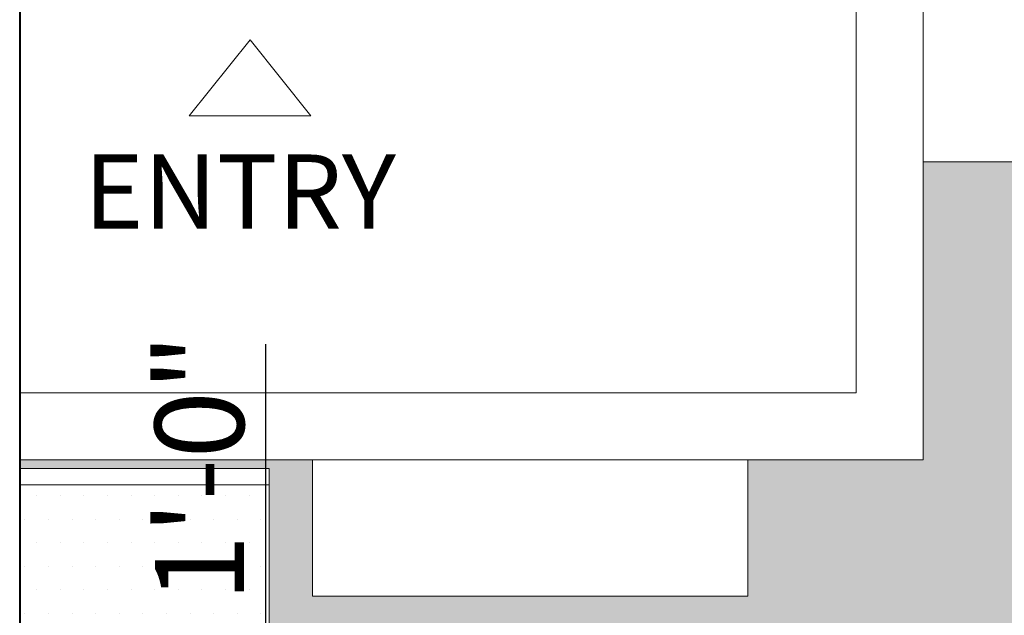
# Model space of a CAD drawing. Units: inches. Extents: x 459864 to 460310, y 324185 to 324787.
# Tile 44 of 112: x 460061 to 460127, y 324242 to 324282. Entities that reach past the tile are written whole.
import ezdxf

# ---------------------------------------------------------------- set-up
doc = ezdxf.new("R2010")
doc.units = ezdxf.units.IN
for name, color, linetype, lineweight in [('A-ANNO-DIMS', 2, 'Continuous', 18), ('A-ANNO-SYMB', 7, 'Continuous', 18), ('A-ANNO-TEXT', 7, 'Continuous', 18), ('A-WALL', 7, 'Continuous', 40), ('L-HRDS', 9, 'Continuous', 18), ('L-PLNT', 3, 'Continuous', 13), ('L-SITE-PATT', 252, 'Continuous', 13)]:
    doc.layers.add(name, color=color, linetype=linetype, lineweight=lineweight)
doc.styles.get("Standard").update_dxf_attribs({"font": 'arial.ttf'})
doc.dimstyles.new('ISO-25', dxfattribs={"dimtxt": 6, "dimasz": 2.5, "dimexe": 1.25, "dimexo": 0.625, "dimtad": 1, "dimdec": 1, "dimlunit": 3, "dimtxsty": 'Standard', "dimcen": 2.5, "dimadec": 0, "dimazin": 0, "dimtfac": 1, "dimtdec": 1, "dimtmove": 0, "dimatfit": 3, "dimfxl": 1, "dimarcsym": 0})

# ---------------------------------------------------------------- blocks, each defined once
blk = doc.blocks.new('*D28')
at = {"layer": 'A-ANNO-DIMS', "color": 0, "lineweight": -2, "transparency": 16777216}
for p, q in [((460148.65, 324370.7), (460136.025, 324370.7)), ((460137.275, 324368.2), (460137.275, 324293.2)), ((460148.65, 324290.7), (460136.025, 324290.7)), ((460137.275, 324290.7), (460137.275, 324198.69))]:
    blk.add_line(p, q, dxfattribs=at)
at = {"layer": 'A-ANNO-DIMS', "color": 0, "transparency": 16777216}
for points in [[(460136.858, 324368.2), (460137.692, 324368.2), (460137.275, 324370.7)], [(460136.858, 324293.2), (460137.692, 324293.2), (460137.275, 324290.7)]]:
    blk.add_solid(points, dxfattribs=at)
at = {"layer": 'Defpoints', "color": 0, "transparency": 16777216}
for p in [(460149.275, 324370.7), (460137.275, 324290.7), (460149.275, 324290.7)]:
    blk.add_point(p, dxfattribs=at)
at = {"layer": 'A-ANNO-DIMS', "color": 0, "transparency": 16777216, "insert": (460133.363, 324243.445), "char_height": 6, "attachment_point": 5, "rotation": 90}
blk.add_mtext('QUEEN BED 6\'-8" TYP.', dxfattribs=at)
blk = doc.blocks.new('*D37')
at = {"layer": 'A-ANNO-DIMS', "color": 0, "lineweight": -2, "transparency": 16777216}
for p, q in [((460077.678, 324241.122), (460077.678, 324260.257)), ((460076.501, 324241.122), (460078.928, 324241.122)), ((460077.678, 324231.608), (460077.678, 324238.622)), ((460076.501, 324229.108), (460078.928, 324229.108))]:
    blk.add_line(p, q, dxfattribs=at)
at = {"layer": 'A-ANNO-DIMS', "color": 0, "transparency": 16777216}
for points in [[(460077.261, 324238.622), (460078.095, 324238.622), (460077.678, 324241.122)], [(460077.261, 324231.608), (460078.095, 324231.608), (460077.678, 324229.108)]]:
    blk.add_solid(points, dxfattribs=at)
at = {"layer": 'Defpoints', "color": 0, "transparency": 16777216}
for p in [(460075.876, 324241.122), (460077.678, 324241.122), (460075.876, 324229.108)]:
    blk.add_point(p, dxfattribs=at)
at = {"layer": 'A-ANNO-DIMS', "color": 0, "transparency": 16777216, "insert": (460073.989, 324251.94), "char_height": 6, "attachment_point": 5, "rotation": 90}
blk.add_mtext('1\'-0"', dxfattribs=at)

msp = doc.modelspace()

# ---------------------------------------------------------------- hatches: boundary and pattern name
at = {"layer": 'L-SITE-PATT'}
h = msp.add_hatch(dxfattribs=at)
h.set_pattern_fill('DOTS', color=256)
h.paths.add_polyline_path([(460269.804, 324283.483), (460247.115, 324283.483), (460121.929, 324283.483), (460121.929, 324252.473), (460117.429, 324252.473), (460110.124, 324252.473), (460110.124, 324243.287), (460080.83, 324243.287), (460080.83, 324252.473), (460061.115, 324252.473), (460061.115, 324251.882), (460077.909, 324251.882), (460077.909, 324199.483), (460080.83, 324199.483), (460080.83, 324207.553), (460110.124, 324207.553), (460110.124, 324199.483), (460110.813, 324199.483), (460262.115, 324199.483), (460269.804, 324199.483)], flags=17)
edge = h.paths.add_edge_path(flags=0)
edge.add_ellipse((460222.59, 324263.813), major_axis=(-8.485, 8.485), ratio=1, start_angle=405, end_angle=495, ccw=False)
edge.add_line((460214.821, 324254.66), (460214.832, 324254.666))
edge.add_ellipse((460222.59, 324263.813), major_axis=(-8.485, 8.485), ratio=1, start_angle=405, end_angle=495, ccw=False)
edge.add_line((460210.759, 324261.781), (460210.768, 324261.787))
edge.add_ellipse((460222.59, 324263.813), major_axis=(-8.485, 8.485), ratio=1, start_angle=405, end_angle=495, ccw=False)
edge.add_ellipse((460222.59, 324263.813), major_axis=(-8.485, 8.485), ratio=1, start_angle=392.75402, end_angle=405, ccw=False)
edge.add_ellipse((460222.59, 324263.813), major_axis=(-8.485, 8.485), ratio=1, start_angle=380.93472, end_angle=392.75402, ccw=False)
edge.add_line((460211.337, 324267.985), (460211.34, 324267.985))
edge.add_ellipse((460222.59, 324263.813), major_axis=(-8.485, 8.485), ratio=1, start_angle=380.93472, end_angle=392.75402, ccw=False)
edge.add_ellipse((460222.59, 324263.813), major_axis=(-8.485, 8.485), ratio=1, start_angle=347.90152, end_angle=380.93472, ccw=False)
edge.add_ellipse((460222.59, 324263.813), major_axis=(-8.485, 8.485), ratio=1, start_angle=327.06192, end_angle=347.90152, ccw=False)
edge.add_ellipse((460222.59, 324263.813), major_axis=(-8.485, 8.485), ratio=1, start_angle=278.32464, end_angle=327.06192, ccw=False)
edge.add_line((460225.158, 324275.536), (460225.158, 324275.535))
edge.add_ellipse((460222.59, 324263.813), major_axis=(-8.485, 8.485), ratio=1, start_angle=278.32464, end_angle=327.06192, ccw=False)
edge.add_ellipse((460222.59, 324263.813), major_axis=(-8.485, 8.485), ratio=1, start_angle=260.64357, end_angle=278.32464, ccw=False)
edge.add_ellipse((460222.59, 324263.813), major_axis=(-8.485, 8.485), ratio=1, start_angle=225, end_angle=260.64357, ccw=False)
edge.add_line((460234.509, 324265.243), (460234.501, 324265.239))
edge.add_ellipse((460222.59, 324263.813), major_axis=(-8.485, 8.485), ratio=1, start_angle=225, end_angle=260.64357, ccw=False)
edge.add_ellipse((460222.59, 324263.813), major_axis=(-8.485, 8.485), ratio=1, start_angle=495, end_angle=585, ccw=False)
edge.add_line((460234.437, 324261.861), (460234.424, 324261.858))
edge.add_ellipse((460222.59, 324263.813), major_axis=(-8.485, 8.485), ratio=1, start_angle=495, end_angle=585, ccw=False)
edge.add_line((460227.95, 324253.067), (460227.946, 324253.083))
edge.add_ellipse((460222.59, 324263.813), major_axis=(-8.485, 8.485), ratio=1, start_angle=495, end_angle=585, ccw=False)
edge.add_line((460226.223, 324252.369), (460226.211, 324252.38))
edge.add_ellipse((460222.59, 324263.813), major_axis=(-8.485, 8.485), ratio=1, start_angle=495, end_angle=585, ccw=False)
h.paths.add_polyline_path([(460219.651, 324254.347), (460218.461, 324253.545), (460218.275, 324254.789), (460219.642, 324256.542), (460219.625, 324260.848), (460216.11, 324257.333), (460214.35, 324256.978), (460215.416, 324259.356), (460212.524, 324258.496), (460213.137, 324259.93), (460218.507, 324263.813), (460222.59, 324263.813), (460222.59, 324267.807), (460218.176, 324272.212), (460219.026, 324274.639), (460222.59, 324272.811), (460222.59, 324275.423), (460223.057, 324274.825), (460222.675, 324273.492), (460225.912, 324267.135), (460219.625, 324260.848)], flags=0)
edge = h.paths.add_edge_path(flags=0)
edge.add_ellipse((460194.576, 324264.046), major_axis=(-8.485, 8.485), ratio=1, start_angle=495, end_angle=585, ccw=False)
edge.add_line((460199.936, 324253.3), (460199.932, 324253.316))
edge.add_ellipse((460194.576, 324264.046), major_axis=(-8.485, 8.485), ratio=1, start_angle=495, end_angle=585, ccw=False)
edge.add_line((460198.208, 324252.603), (460198.196, 324252.613))
edge.add_ellipse((460194.576, 324264.046), major_axis=(-8.485, 8.485), ratio=1, start_angle=495, end_angle=585, ccw=False)
edge.add_ellipse((460194.576, 324264.046), major_axis=(-8.485, 8.485), ratio=1, start_angle=405, end_angle=495, ccw=False)
edge.add_line((460186.806, 324254.893), (460186.817, 324254.899))
edge.add_ellipse((460194.576, 324264.046), major_axis=(-8.485, 8.485), ratio=1, start_angle=405, end_angle=495, ccw=False)
edge.add_line((460182.744, 324262.014), (460182.753, 324262.02))
edge.add_ellipse((460194.576, 324264.046), major_axis=(-8.485, 8.485), ratio=1, start_angle=405, end_angle=495, ccw=False)
edge.add_ellipse((460194.576, 324264.046), major_axis=(-8.485, 8.485), ratio=1, start_angle=392.75402, end_angle=405, ccw=False)
edge.add_ellipse((460194.576, 324264.046), major_axis=(-8.485, 8.485), ratio=1, start_angle=380.93472, end_angle=392.75402, ccw=False)
edge.add_line((460183.323, 324268.218), (460183.326, 324268.218))
edge.add_ellipse((460194.576, 324264.046), major_axis=(-8.485, 8.485), ratio=1, start_angle=380.93472, end_angle=392.75402, ccw=False)
edge.add_ellipse((460194.576, 324264.046), major_axis=(-8.485, 8.485), ratio=1, start_angle=347.90152, end_angle=380.93472, ccw=False)
edge.add_ellipse((460194.576, 324264.046), major_axis=(-8.485, 8.485), ratio=1, start_angle=327.06192, end_angle=347.90152, ccw=False)
edge.add_ellipse((460194.576, 324264.046), major_axis=(-8.485, 8.485), ratio=1, start_angle=278.32464, end_angle=327.06192, ccw=False)
edge.add_line((460197.144, 324275.769), (460197.143, 324275.768))
edge.add_ellipse((460194.576, 324264.046), major_axis=(-8.485, 8.485), ratio=1, start_angle=278.32464, end_angle=327.06192, ccw=False)
edge.add_ellipse((460194.576, 324264.046), major_axis=(-8.485, 8.485), ratio=1, start_angle=260.64357, end_angle=278.32464, ccw=False)
edge.add_ellipse((460194.576, 324264.046), major_axis=(-8.485, 8.485), ratio=1, start_angle=225, end_angle=260.64357, ccw=False)
edge.add_line((460206.494, 324265.476), (460206.487, 324265.473))
edge.add_ellipse((460194.576, 324264.046), major_axis=(-8.485, 8.485), ratio=1, start_angle=225, end_angle=260.64357, ccw=False)
edge.add_ellipse((460194.576, 324264.046), major_axis=(-8.485, 8.485), ratio=1, start_angle=495, end_angle=585, ccw=False)
edge.add_line((460206.422, 324262.094), (460206.409, 324262.091))
h.paths.add_polyline_path([(460191.61, 324261.081), (460191.637, 324254.58), (460190.447, 324253.778), (460190.261, 324255.023), (460191.628, 324256.775), (460191.61, 324261.081), (460188.096, 324257.566), (460186.335, 324257.211), (460187.402, 324259.589), (460184.509, 324258.729), (460185.123, 324260.163), (460190.493, 324264.046), (460194.576, 324264.046), (460194.576, 324268.04), (460190.161, 324272.446), (460191.011, 324274.872), (460194.576, 324273.044), (460194.576, 324275.657), (460195.043, 324275.058), (460194.661, 324273.725), (460197.897, 324267.368)], flags=0)
edge = h.paths.add_edge_path(flags=0)
edge.add_ellipse((460252.912, 324263.578), major_axis=(-8.485, 8.485), ratio=1, start_angle=405, end_angle=495, ccw=False)
edge.add_line((460241.081, 324261.545), (460241.089, 324261.551))
edge.add_ellipse((460252.912, 324263.578), major_axis=(-8.485, 8.485), ratio=1, start_angle=405, end_angle=495, ccw=False)
edge.add_ellipse((460252.912, 324263.578), major_axis=(-8.485, 8.485), ratio=1, start_angle=392.75402, end_angle=405, ccw=False)
edge.add_ellipse((460252.912, 324263.578), major_axis=(-8.485, 8.485), ratio=1, start_angle=380.93472, end_angle=392.75402, ccw=False)
edge.add_line((460241.659, 324267.749), (460241.662, 324267.749))
edge.add_ellipse((460252.912, 324263.578), major_axis=(-8.485, 8.485), ratio=1, start_angle=380.93472, end_angle=392.75402, ccw=False)
edge.add_ellipse((460252.912, 324263.578), major_axis=(-8.485, 8.485), ratio=1, start_angle=347.90152, end_angle=380.93472, ccw=False)
edge.add_ellipse((460252.912, 324263.578), major_axis=(-8.485, 8.485), ratio=1, start_angle=327.06192, end_angle=347.90152, ccw=False)
edge.add_ellipse((460252.912, 324263.578), major_axis=(-8.485, 8.485), ratio=1, start_angle=278.32464, end_angle=327.06192, ccw=False)
edge.add_line((460255.48, 324275.3), (460255.479, 324275.299))
edge.add_ellipse((460252.912, 324263.578), major_axis=(-8.485, 8.485), ratio=1, start_angle=278.32464, end_angle=327.06192, ccw=False)
edge.add_ellipse((460252.912, 324263.578), major_axis=(-8.485, 8.485), ratio=1, start_angle=260.64357, end_angle=278.32464, ccw=False)
edge.add_ellipse((460252.912, 324263.578), major_axis=(-8.485, 8.485), ratio=1, start_angle=225, end_angle=260.64357, ccw=False)
edge.add_line((460264.83, 324265.007), (460264.823, 324265.004))
edge.add_ellipse((460252.912, 324263.578), major_axis=(-8.485, 8.485), ratio=1, start_angle=225, end_angle=260.64357, ccw=False)
edge.add_ellipse((460252.912, 324263.578), major_axis=(-8.485, 8.485), ratio=1, start_angle=495, end_angle=585, ccw=False)
edge.add_line((460264.758, 324261.626), (460264.745, 324261.622))
edge.add_ellipse((460252.912, 324263.578), major_axis=(-8.485, 8.485), ratio=1, start_angle=495, end_angle=585, ccw=False)
edge.add_line((460258.272, 324252.832), (460258.268, 324252.848))
edge.add_ellipse((460252.912, 324263.578), major_axis=(-8.485, 8.485), ratio=1, start_angle=495, end_angle=585, ccw=False)
edge.add_line((460256.545, 324252.134), (460256.533, 324252.144))
edge.add_ellipse((460252.912, 324263.578), major_axis=(-8.485, 8.485), ratio=1, start_angle=495, end_angle=585, ccw=False)
edge.add_ellipse((460252.912, 324263.578), major_axis=(-8.485, 8.485), ratio=1, start_angle=405, end_angle=495, ccw=False)
edge.add_line((460245.143, 324254.424), (460245.153, 324254.43))
h.paths.add_polyline_path([(460244.672, 324256.742), (460245.738, 324259.12), (460242.846, 324258.26), (460243.459, 324259.694), (460248.829, 324263.578), (460252.912, 324263.578), (460252.912, 324267.571), (460248.497, 324271.977), (460249.348, 324274.403), (460252.912, 324272.576), (460252.912, 324275.188), (460253.379, 324274.589), (460252.997, 324273.257), (460256.233, 324266.899), (460249.946, 324260.612), (460249.973, 324254.111), (460248.783, 324253.309), (460248.597, 324254.554), (460249.964, 324256.306), (460249.946, 324260.612), (460246.432, 324257.097)], flags=0)
edge = h.paths.add_edge_path(flags=0)
edge.add_ellipse((460167.439, 324262.833), major_axis=(-8.485, 8.485), ratio=1, start_angle=495, end_angle=585, ccw=False)
edge.add_line((460172.799, 324252.087), (460172.795, 324252.103))
edge.add_ellipse((460167.439, 324262.833), major_axis=(-8.485, 8.485), ratio=1, start_angle=495, end_angle=585, ccw=False)
edge.add_line((460171.071, 324251.389), (460171.059, 324251.399))
edge.add_ellipse((460167.439, 324262.833), major_axis=(-8.485, 8.485), ratio=1, start_angle=495, end_angle=585, ccw=False)
edge.add_ellipse((460167.439, 324262.833), major_axis=(-8.485, 8.485), ratio=1, start_angle=405, end_angle=495, ccw=False)
edge.add_line((460159.669, 324253.679), (460159.68, 324253.685))
edge.add_ellipse((460167.439, 324262.833), major_axis=(-8.485, 8.485), ratio=1, start_angle=405, end_angle=495, ccw=False)
edge.add_line((460155.607, 324260.8), (460155.616, 324260.806))
edge.add_ellipse((460167.439, 324262.833), major_axis=(-8.485, 8.485), ratio=1, start_angle=405, end_angle=495, ccw=False)
edge.add_ellipse((460167.439, 324262.833), major_axis=(-8.485, 8.485), ratio=1, start_angle=392.75402, end_angle=405, ccw=False)
edge.add_ellipse((460167.439, 324262.833), major_axis=(-8.485, 8.485), ratio=1, start_angle=380.93472, end_angle=392.75402, ccw=False)
edge.add_line((460156.185, 324267.005), (460156.189, 324267.005))
edge.add_ellipse((460167.439, 324262.833), major_axis=(-8.485, 8.485), ratio=1, start_angle=380.93472, end_angle=392.75402, ccw=False)
edge.add_ellipse((460167.439, 324262.833), major_axis=(-8.485, 8.485), ratio=1, start_angle=347.90152, end_angle=380.93472, ccw=False)
edge.add_ellipse((460167.439, 324262.833), major_axis=(-8.485, 8.485), ratio=1, start_angle=327.06192, end_angle=347.90152, ccw=False)
edge.add_ellipse((460167.439, 324262.833), major_axis=(-8.485, 8.485), ratio=1, start_angle=278.32464, end_angle=327.06192, ccw=False)
edge.add_line((460170.007, 324274.556), (460170.006, 324274.554))
edge.add_ellipse((460167.439, 324262.833), major_axis=(-8.485, 8.485), ratio=1, start_angle=278.32464, end_angle=327.06192, ccw=False)
edge.add_ellipse((460167.439, 324262.833), major_axis=(-8.485, 8.485), ratio=1, start_angle=260.64357, end_angle=278.32464, ccw=False)
edge.add_ellipse((460167.439, 324262.833), major_axis=(-8.485, 8.485), ratio=1, start_angle=225, end_angle=260.64357, ccw=False)
edge.add_line((460179.357, 324264.262), (460179.35, 324264.259))
edge.add_ellipse((460167.439, 324262.833), major_axis=(-8.485, 8.485), ratio=1, start_angle=225, end_angle=260.64357, ccw=False)
edge.add_ellipse((460167.439, 324262.833), major_axis=(-8.485, 8.485), ratio=1, start_angle=495, end_angle=585, ccw=False)
edge.add_line((460179.285, 324260.881), (460179.272, 324260.877))
h.paths.add_polyline_path([(460164.473, 324259.867), (460164.5, 324253.366), (460163.31, 324252.565), (460163.124, 324253.809), (460164.491, 324255.561), (460164.473, 324259.867), (460160.958, 324256.353), (460159.198, 324255.998), (460160.265, 324258.375), (460157.372, 324257.515), (460157.986, 324258.949), (460163.356, 324262.833), (460167.439, 324262.833), (460167.439, 324266.826), (460163.024, 324271.232), (460163.874, 324273.659), (460167.439, 324271.831), (460167.439, 324274.443), (460167.905, 324273.844), (460167.524, 324272.512), (460170.76, 324266.154)], flags=0)
edge = h.paths.add_edge_path(flags=0)
edge.add_ellipse((460140.758, 324262.37), major_axis=(-8.485, 8.485), ratio=1, start_angle=495, end_angle=585, ccw=False)
edge.add_line((460146.118, 324251.624), (460146.114, 324251.639))
edge.add_ellipse((460140.758, 324262.37), major_axis=(-8.485, 8.485), ratio=1, start_angle=495, end_angle=585, ccw=False)
edge.add_line((460144.391, 324250.926), (460144.379, 324250.936))
edge.add_ellipse((460140.758, 324262.37), major_axis=(-8.485, 8.485), ratio=1, start_angle=495, end_angle=585, ccw=False)
edge.add_ellipse((460140.758, 324262.37), major_axis=(-8.485, 8.485), ratio=1, start_angle=405, end_angle=495, ccw=False)
edge.add_line((460132.989, 324253.216), (460132.999, 324253.222))
edge.add_ellipse((460140.758, 324262.37), major_axis=(-8.485, 8.485), ratio=1, start_angle=405, end_angle=495, ccw=False)
edge.add_line((460128.927, 324260.337), (460128.935, 324260.343))
edge.add_ellipse((460140.758, 324262.37), major_axis=(-8.485, 8.485), ratio=1, start_angle=405, end_angle=495, ccw=False)
edge.add_ellipse((460140.758, 324262.37), major_axis=(-8.485, 8.485), ratio=1, start_angle=392.75402, end_angle=405, ccw=False)
edge.add_ellipse((460140.758, 324262.37), major_axis=(-8.485, 8.485), ratio=1, start_angle=380.93472, end_angle=392.75402, ccw=False)
edge.add_line((460129.505, 324266.541), (460129.508, 324266.541))
edge.add_ellipse((460140.758, 324262.37), major_axis=(-8.485, 8.485), ratio=1, start_angle=380.93472, end_angle=392.75402, ccw=False)
edge.add_ellipse((460140.758, 324262.37), major_axis=(-8.485, 8.485), ratio=1, start_angle=347.90152, end_angle=380.93472, ccw=False)
edge.add_ellipse((460140.758, 324262.37), major_axis=(-8.485, 8.485), ratio=1, start_angle=327.06192, end_angle=347.90152, ccw=False)
edge.add_ellipse((460140.758, 324262.37), major_axis=(-8.485, 8.485), ratio=1, start_angle=278.32464, end_angle=327.06192, ccw=False)
edge.add_line((460143.326, 324274.092), (460143.325, 324274.091))
edge.add_ellipse((460140.758, 324262.37), major_axis=(-8.485, 8.485), ratio=1, start_angle=278.32464, end_angle=327.06192, ccw=False)
edge.add_ellipse((460140.758, 324262.37), major_axis=(-8.485, 8.485), ratio=1, start_angle=260.64357, end_angle=278.32464, ccw=False)
edge.add_ellipse((460140.758, 324262.37), major_axis=(-8.485, 8.485), ratio=1, start_angle=225, end_angle=260.64357, ccw=False)
edge.add_line((460152.677, 324263.799), (460152.669, 324263.796))
edge.add_ellipse((460140.758, 324262.37), major_axis=(-8.485, 8.485), ratio=1, start_angle=225, end_angle=260.64357, ccw=False)
edge.add_ellipse((460140.758, 324262.37), major_axis=(-8.485, 8.485), ratio=1, start_angle=495, end_angle=585, ccw=False)
edge.add_line((460152.604, 324260.418), (460152.592, 324260.414))
h.paths.add_polyline_path([(460137.792, 324259.404), (460137.819, 324252.903), (460136.629, 324252.101), (460136.443, 324253.346), (460137.81, 324255.098), (460137.792, 324259.404), (460134.278, 324255.889), (460132.518, 324255.534), (460133.584, 324257.912), (460130.692, 324257.052), (460131.305, 324258.486), (460136.675, 324262.37), (460140.758, 324262.37), (460140.758, 324266.363), (460136.343, 324270.769), (460137.194, 324273.195), (460140.758, 324271.367), (460140.758, 324273.98), (460141.225, 324273.381), (460140.843, 324272.049), (460144.079, 324265.691)], flags=0)
h.paths.add_polyline_path([(460110.124, 324227.414), (460080.83, 324227.414), (460080.83, 324235.484), (460110.124, 324235.484)], flags=16)
h.paths.add_polyline_path([(460110.124, 324220.797), (460110.124, 324212.727), (460080.83, 324212.727), (460080.83, 324220.797)], flags=16)
h.paths.add_polyline_path([(460269.804, 324283.483), (460247.115, 324283.483), (460121.929, 324283.483), (460121.929, 324252.473), (460117.429, 324252.473), (460110.124, 324252.473), (460110.124, 324243.287), (460080.83, 324243.287), (460080.83, 324252.473), (460061.115, 324252.473), (460061.115, 324251.882), (460077.909, 324251.882), (460077.909, 324199.483), (460080.83, 324199.483), (460080.83, 324207.553), (460110.124, 324207.553), (460110.124, 324199.483), (460262.115, 324199.483), (460269.804, 324199.483)], flags=17)
h.paths.add_polyline_path([(460219.651, 324254.347), (460218.461, 324253.545), (460218.275, 324254.789), (460219.642, 324256.542), (460219.625, 324260.848), (460216.11, 324257.333), (460214.35, 324256.978), (460215.416, 324259.356), (460212.524, 324258.496), (460213.137, 324259.93), (460218.507, 324263.813), (460222.59, 324263.813), (460220.18, 324266.223), (460215.461, 324265.308), (460211.835, 324266.137), (460216.247, 324267.985), (460218.418, 324267.985), (460222.59, 324263.813), (460222.59, 324267.807), (460218.176, 324272.212), (460219.026, 324274.639), (460222.59, 324272.811), (460222.59, 324275.423), (460223.057, 324274.825), (460222.675, 324273.492), (460225.912, 324267.135), (460222.59, 324263.813), (460231.383, 324263.813), (460228.485, 324262.488), (460224.425, 324261.978), (460228.68, 324257.724), (460228.966, 324254.791), (460227.142, 324256.537), (460227.542, 324254.819), (460227.333, 324253.614), (460222.59, 324259.985), (460222.59, 324255.497), (460221.377, 324256.541), (460220.576, 324261.799), (460219.625, 324260.848)], flags=0)
h.paths.add_polyline_path([(460199.127, 324256.77), (460199.528, 324255.052), (460199.319, 324253.848), (460194.576, 324260.218), (460194.576, 324255.73), (460193.363, 324256.774), (460192.561, 324262.032), (460191.61, 324261.081), (460191.637, 324254.58), (460190.447, 324253.778), (460190.261, 324255.023), (460191.628, 324256.775), (460191.61, 324261.081), (460188.096, 324257.566), (460186.335, 324257.211), (460187.402, 324259.589), (460184.509, 324258.729), (460185.123, 324260.163), (460190.493, 324264.046), (460194.576, 324264.046), (460192.166, 324266.456), (460187.446, 324265.541), (460183.82, 324266.37), (460188.232, 324268.218), (460190.404, 324268.218), (460194.576, 324264.046), (460194.576, 324268.04), (460190.161, 324272.446), (460191.011, 324274.872), (460194.576, 324273.044), (460194.576, 324275.657), (460195.043, 324275.058), (460194.661, 324273.725), (460197.897, 324267.368), (460194.576, 324264.046), (460203.368, 324264.046), (460200.47, 324262.721), (460196.411, 324262.212), (460200.665, 324257.957), (460200.951, 324255.024)], flags=0)
h.paths.add_polyline_path([(460244.672, 324256.742), (460245.738, 324259.12), (460242.846, 324258.26), (460243.459, 324259.694), (460248.829, 324263.578), (460252.912, 324263.578), (460250.502, 324265.987), (460245.783, 324265.072), (460242.156, 324265.901), (460246.568, 324267.749), (460248.74, 324267.749), (460252.912, 324263.578), (460252.912, 324267.571), (460248.497, 324271.977), (460249.348, 324274.403), (460252.912, 324272.576), (460252.912, 324275.188), (460253.379, 324274.589), (460252.997, 324273.257), (460256.233, 324266.899), (460252.912, 324263.578), (460261.705, 324263.578), (460258.806, 324262.252), (460254.747, 324261.743), (460259.002, 324257.488), (460259.288, 324254.555), (460257.463, 324256.301), (460257.864, 324254.583), (460257.655, 324253.379), (460252.912, 324259.749), (460252.912, 324255.261), (460251.699, 324256.305), (460250.897, 324261.563), (460249.946, 324260.612), (460249.973, 324254.111), (460248.783, 324253.309), (460248.597, 324254.554), (460249.964, 324256.306), (460249.946, 324260.612), (460246.432, 324257.097)], flags=0)
h.paths.add_polyline_path([(460173.528, 324256.743), (460173.814, 324253.811), (460171.99, 324255.556), (460172.39, 324253.838), (460172.182, 324252.634), (460167.439, 324259.004), (460167.439, 324254.516), (460166.226, 324255.56), (460165.424, 324260.818), (460164.473, 324259.867), (460164.5, 324253.366), (460163.31, 324252.565), (460163.124, 324253.809), (460164.491, 324255.561), (460164.473, 324259.867), (460160.958, 324256.353), (460159.198, 324255.998), (460160.265, 324258.375), (460157.372, 324257.515), (460157.986, 324258.949), (460163.356, 324262.833), (460167.439, 324262.833), (460165.029, 324265.243), (460160.309, 324264.327), (460156.683, 324265.156), (460161.095, 324267.005), (460163.267, 324267.005), (460167.439, 324262.833), (460167.439, 324266.826), (460163.024, 324271.232), (460163.874, 324273.659), (460167.439, 324271.831), (460167.439, 324274.443), (460167.905, 324273.844), (460167.524, 324272.512), (460170.76, 324266.154), (460167.439, 324262.833), (460176.231, 324262.833), (460173.333, 324261.507), (460169.274, 324260.998)], flags=0)
h.paths.add_polyline_path([(460146.848, 324256.28), (460147.134, 324253.347), (460145.31, 324255.093), (460145.71, 324253.375), (460145.501, 324252.171), (460140.758, 324258.541), (460140.758, 324254.053), (460139.545, 324255.097), (460138.744, 324260.355), (460137.792, 324259.404), (460137.819, 324252.903), (460136.629, 324252.101), (460136.443, 324253.346), (460137.81, 324255.098), (460137.792, 324259.404), (460134.278, 324255.889), (460132.518, 324255.534), (460133.584, 324257.912), (460130.692, 324257.052), (460131.305, 324258.486), (460136.675, 324262.37), (460140.758, 324262.37), (460138.348, 324264.779), (460133.629, 324263.864), (460130.002, 324264.693), (460134.414, 324266.541), (460136.586, 324266.541), (460140.758, 324262.37), (460140.758, 324266.363), (460136.343, 324270.769), (460137.194, 324273.195), (460140.758, 324271.367), (460140.758, 324273.98), (460141.225, 324273.381), (460140.843, 324272.049), (460144.079, 324265.691), (460140.758, 324262.37), (460149.551, 324262.37), (460146.653, 324261.044), (460142.593, 324260.535)], flags=0)
edge = h.paths.add_edge_path()
edge.add_line((460269.804, 324272.549), (460260.881, 324272.549))
edge.add_ellipse((460252.912, 324263.578), major_axis=(-8.485, 8.485), ratio=1, start_angle=260.64357, end_angle=273.38462, ccw=False)
edge.add_line((460262.283, 324271.092), (460262.261, 324271.091))
edge.add_ellipse((460252.912, 324263.578), major_axis=(-8.485, 8.485), ratio=1, start_angle=260.64357, end_angle=273.38462, ccw=False)
edge.add_ellipse((460252.912, 324263.578), major_axis=(-8.485, 8.485), ratio=1, start_angle=225, end_angle=260.64357, ccw=False)
edge.add_line((460263.609, 324269.063), (460263.572, 324269.058))
edge.add_ellipse((460252.912, 324263.578), major_axis=(-8.485, 8.485), ratio=1, start_angle=225, end_angle=260.64357, ccw=False)
edge.add_line((460264.615, 324266.306), (460264.585, 324266.305))
edge.add_ellipse((460252.912, 324263.578), major_axis=(-8.485, 8.485), ratio=1, start_angle=225, end_angle=260.64357, ccw=False)
edge.add_line((460264.83, 324265.007), (460264.823, 324265.004))
edge.add_ellipse((460252.912, 324263.578), major_axis=(-8.485, 8.485), ratio=1, start_angle=225, end_angle=260.64357, ccw=False)
edge.add_ellipse((460252.912, 324263.578), major_axis=(-8.485, 8.485), ratio=1, start_angle=495, end_angle=585, ccw=False)
edge.add_line((460264.758, 324261.626), (460264.745, 324261.622))
edge.add_ellipse((460252.912, 324263.578), major_axis=(-8.485, 8.485), ratio=1, start_angle=495, end_angle=585, ccw=False)
edge.add_line((460263.442, 324257.739), (460263.389, 324257.779))
edge.add_ellipse((460252.912, 324263.578), major_axis=(-8.485, 8.485), ratio=1, start_angle=495, end_angle=585, ccw=False)
edge.add_line((460258.128, 324252.744), (460258.102, 324252.779))
edge.add_ellipse((460252.912, 324263.578), major_axis=(-8.485, 8.485), ratio=1, start_angle=495, end_angle=585, ccw=False)
edge.add_line((460256.545, 324252.134), (460256.533, 324252.144))
edge.add_ellipse((460252.912, 324263.578), major_axis=(-8.485, 8.485), ratio=1, start_angle=495, end_angle=585, ccw=False)
edge.add_ellipse((460252.912, 324263.578), major_axis=(-8.485, 8.485), ratio=1, start_angle=405, end_angle=495, ccw=False)
edge.add_line((460250.594, 324251.78), (460250.605, 324251.82))
edge.add_ellipse((460252.912, 324263.578), major_axis=(-8.485, 8.485), ratio=1, start_angle=405, end_angle=495, ccw=False)
edge.add_line((460245.143, 324254.424), (460245.153, 324254.43))
edge.add_ellipse((460252.912, 324263.578), major_axis=(-8.485, 8.485), ratio=1, start_angle=405, end_angle=495, ccw=False)
edge.add_line((460243.525, 324256.059), (460243.56, 324256.091))
edge.add_ellipse((460252.912, 324263.578), major_axis=(-8.485, 8.485), ratio=1, start_angle=405, end_angle=495, ccw=False)
edge.add_line((460241.44, 324259.893), (460241.522, 324259.896))
edge.add_ellipse((460252.912, 324263.578), major_axis=(-8.485, 8.485), ratio=1, start_angle=405, end_angle=495, ccw=False)
edge.add_line((460241.081, 324261.545), (460241.089, 324261.551))
edge.add_ellipse((460252.912, 324263.578), major_axis=(-8.485, 8.485), ratio=1, start_angle=405, end_angle=495, ccw=False)
edge.add_ellipse((460252.912, 324263.578), major_axis=(-8.485, 8.485), ratio=1, start_angle=392.75402, end_angle=405, ccw=False)
edge.add_line((460241.05, 324265.438), (460241.063, 324265.443))
edge.add_ellipse((460252.912, 324263.578), major_axis=(-8.485, 8.485), ratio=1, start_angle=392.75402, end_angle=405, ccw=False)
edge.add_ellipse((460252.912, 324263.578), major_axis=(-8.485, 8.485), ratio=1, start_angle=380.93472, end_angle=392.75402, ccw=False)
edge.add_line((460241.452, 324267.176), (460241.469, 324267.171))
edge.add_ellipse((460252.912, 324263.578), major_axis=(-8.485, 8.485), ratio=1, start_angle=380.93472, end_angle=392.75402, ccw=False)
edge.add_line((460241.659, 324267.749), (460241.662, 324267.749))
edge.add_ellipse((460252.912, 324263.578), major_axis=(-8.485, 8.485), ratio=1, start_angle=380.93472, end_angle=392.75402, ccw=False)
edge.add_ellipse((460252.912, 324263.578), major_axis=(-8.485, 8.485), ratio=1, start_angle=356.61538, end_angle=380.93472, ccw=False)
edge.add_line((460244.88, 324272.488), (460244.713, 324272.549))
edge.add_line((460244.713, 324272.549), (460230.817, 324272.549))
edge.add_ellipse((460222.59, 324263.813), major_axis=(-8.485, 8.485), ratio=1, start_angle=260.64357, end_angle=271.71777, ccw=False)
edge.add_ellipse((460222.59, 324263.813), major_axis=(-8.485, 8.485), ratio=1, start_angle=225, end_angle=260.64357, ccw=False)
edge.add_line((460233.287, 324269.299), (460233.25, 324269.294))
edge.add_ellipse((460222.59, 324263.813), major_axis=(-8.485, 8.485), ratio=1, start_angle=225, end_angle=260.64357, ccw=False)
edge.add_line((460234.294, 324266.541), (460234.264, 324266.541))
edge.add_ellipse((460222.59, 324263.813), major_axis=(-8.485, 8.485), ratio=1, start_angle=225, end_angle=260.64357, ccw=False)
edge.add_line((460234.509, 324265.243), (460234.501, 324265.239))
edge.add_ellipse((460222.59, 324263.813), major_axis=(-8.485, 8.485), ratio=1, start_angle=225, end_angle=260.64357, ccw=False)
edge.add_ellipse((460222.59, 324263.813), major_axis=(-8.485, 8.485), ratio=1, start_angle=495, end_angle=585, ccw=False)
edge.add_line((460234.437, 324261.861), (460234.424, 324261.858))
edge.add_ellipse((460222.59, 324263.813), major_axis=(-8.485, 8.485), ratio=1, start_angle=495, end_angle=585, ccw=False)
edge.add_line((460233.121, 324257.975), (460233.068, 324258.015))
edge.add_ellipse((460222.59, 324263.813), major_axis=(-8.485, 8.485), ratio=1, start_angle=495, end_angle=585, ccw=False)
edge.add_line((460227.806, 324252.979), (460227.78, 324253.014))
edge.add_ellipse((460222.59, 324263.813), major_axis=(-8.485, 8.485), ratio=1, start_angle=495, end_angle=585, ccw=False)
edge.add_line((460226.223, 324252.369), (460226.211, 324252.38))
edge.add_ellipse((460222.59, 324263.813), major_axis=(-8.485, 8.485), ratio=1, start_angle=495, end_angle=585, ccw=False)
edge.add_ellipse((460222.59, 324263.813), major_axis=(-8.485, 8.485), ratio=1, start_angle=405, end_angle=495, ccw=False)
edge.add_line((460220.272, 324252.016), (460220.283, 324252.055))
edge.add_ellipse((460222.59, 324263.813), major_axis=(-8.485, 8.485), ratio=1, start_angle=405, end_angle=495, ccw=False)
edge.add_line((460214.821, 324254.66), (460214.832, 324254.666))
edge.add_ellipse((460222.59, 324263.813), major_axis=(-8.485, 8.485), ratio=1, start_angle=405, end_angle=495, ccw=False)
edge.add_line((460213.203, 324256.295), (460213.239, 324256.327))
edge.add_ellipse((460222.59, 324263.813), major_axis=(-8.485, 8.485), ratio=1, start_angle=405, end_angle=495, ccw=False)
edge.add_line((460211.118, 324260.128), (460211.201, 324260.131))
edge.add_ellipse((460222.59, 324263.813), major_axis=(-8.485, 8.485), ratio=1, start_angle=405, end_angle=495, ccw=False)
edge.add_line((460210.759, 324261.781), (460210.768, 324261.787))
edge.add_ellipse((460222.59, 324263.813), major_axis=(-8.485, 8.485), ratio=1, start_angle=405, end_angle=495, ccw=False)
edge.add_ellipse((460222.59, 324263.813), major_axis=(-8.485, 8.485), ratio=1, start_angle=392.75402, end_angle=405, ccw=False)
edge.add_line((460210.729, 324265.673), (460210.741, 324265.678))
edge.add_ellipse((460222.59, 324263.813), major_axis=(-8.485, 8.485), ratio=1, start_angle=392.75402, end_angle=405, ccw=False)
edge.add_ellipse((460222.59, 324263.813), major_axis=(-8.485, 8.485), ratio=1, start_angle=380.93472, end_angle=392.75402, ccw=False)
edge.add_line((460211.13, 324267.412), (460211.147, 324267.407))
edge.add_ellipse((460222.59, 324263.813), major_axis=(-8.485, 8.485), ratio=1, start_angle=380.93472, end_angle=392.75402, ccw=False)
edge.add_line((460211.337, 324267.985), (460211.34, 324267.985))
edge.add_ellipse((460222.59, 324263.813), major_axis=(-8.485, 8.485), ratio=1, start_angle=380.93472, end_angle=392.75402, ccw=False)
edge.add_ellipse((460222.59, 324263.813), major_axis=(-8.485, 8.485), ratio=1, start_angle=358.28223, end_angle=380.93472, ccw=False)
edge.add_line((460213.705, 324271.902), (460213.709, 324271.869))
edge.add_ellipse((460222.59, 324263.813), major_axis=(-8.485, 8.485), ratio=1, start_angle=358.28223, end_angle=380.93472, ccw=False)
edge.add_line((460214.363, 324272.549), (460203.078, 324272.549))
edge.add_line((460203.078, 324272.549), (460203.06, 324272.531))
edge.add_ellipse((460194.576, 324264.046), major_axis=(-8.485, 8.485), ratio=1, start_angle=260.64357, end_angle=270.11679, ccw=False)
edge.add_line((460203.957, 324271.561), (460203.921, 324271.56))
edge.add_ellipse((460194.576, 324264.046), major_axis=(-8.485, 8.485), ratio=1, start_angle=260.64357, end_angle=270.11679, ccw=False)
edge.add_ellipse((460194.576, 324264.046), major_axis=(-8.485, 8.485), ratio=1, start_angle=225, end_angle=260.64357, ccw=False)
edge.add_line((460205.272, 324269.532), (460205.235, 324269.527))
edge.add_ellipse((460194.576, 324264.046), major_axis=(-8.485, 8.485), ratio=1, start_angle=225, end_angle=260.64357, ccw=False)
edge.add_line((460206.279, 324266.774), (460206.249, 324266.774))
edge.add_ellipse((460194.576, 324264.046), major_axis=(-8.485, 8.485), ratio=1, start_angle=225, end_angle=260.64357, ccw=False)
edge.add_line((460206.494, 324265.476), (460206.487, 324265.473))
edge.add_ellipse((460194.576, 324264.046), major_axis=(-8.485, 8.485), ratio=1, start_angle=225, end_angle=260.64357, ccw=False)
edge.add_ellipse((460194.576, 324264.046), major_axis=(-8.485, 8.485), ratio=1, start_angle=495, end_angle=585, ccw=False)
edge.add_line((460206.422, 324262.094), (460206.409, 324262.091))
edge.add_ellipse((460194.576, 324264.046), major_axis=(-8.485, 8.485), ratio=1, start_angle=495, end_angle=585, ccw=False)
edge.add_line((460205.106, 324258.208), (460205.053, 324258.248))
edge.add_ellipse((460194.576, 324264.046), major_axis=(-8.485, 8.485), ratio=1, start_angle=495, end_angle=585, ccw=False)
edge.add_line((460199.792, 324253.212), (460199.766, 324253.248))
edge.add_ellipse((460194.576, 324264.046), major_axis=(-8.485, 8.485), ratio=1, start_angle=495, end_angle=585, ccw=False)
edge.add_line((460198.208, 324252.603), (460198.196, 324252.613))
edge.add_ellipse((460194.576, 324264.046), major_axis=(-8.485, 8.485), ratio=1, start_angle=495, end_angle=585, ccw=False)
edge.add_ellipse((460194.576, 324264.046), major_axis=(-8.485, 8.485), ratio=1, start_angle=405, end_angle=495, ccw=False)
edge.add_line((460192.258, 324252.249), (460192.268, 324252.289))
edge.add_ellipse((460194.576, 324264.046), major_axis=(-8.485, 8.485), ratio=1, start_angle=405, end_angle=495, ccw=False)
edge.add_line((460186.806, 324254.893), (460186.817, 324254.899))
edge.add_ellipse((460194.576, 324264.046), major_axis=(-8.485, 8.485), ratio=1, start_angle=405, end_angle=495, ccw=False)
edge.add_line((460185.188, 324256.528), (460185.224, 324256.56))
edge.add_ellipse((460194.576, 324264.046), major_axis=(-8.485, 8.485), ratio=1, start_angle=405, end_angle=495, ccw=False)
edge.add_line((460183.104, 324260.362), (460183.186, 324260.365))
edge.add_ellipse((460194.576, 324264.046), major_axis=(-8.485, 8.485), ratio=1, start_angle=405, end_angle=495, ccw=False)
edge.add_line((460182.744, 324262.014), (460182.753, 324262.02))
edge.add_ellipse((460194.576, 324264.046), major_axis=(-8.485, 8.485), ratio=1, start_angle=405, end_angle=495, ccw=False)
edge.add_ellipse((460194.576, 324264.046), major_axis=(-8.485, 8.485), ratio=1, start_angle=392.75402, end_angle=405, ccw=False)
edge.add_line((460182.714, 324265.906), (460182.726, 324265.912))
edge.add_ellipse((460194.576, 324264.046), major_axis=(-8.485, 8.485), ratio=1, start_angle=392.75402, end_angle=405, ccw=False)
edge.add_ellipse((460194.576, 324264.046), major_axis=(-8.485, 8.485), ratio=1, start_angle=380.93472, end_angle=392.75402, ccw=False)
edge.add_line((460183.116, 324267.645), (460183.133, 324267.64))
edge.add_ellipse((460194.576, 324264.046), major_axis=(-8.485, 8.485), ratio=1, start_angle=380.93472, end_angle=392.75402, ccw=False)
edge.add_line((460183.323, 324268.218), (460183.326, 324268.218))
edge.add_ellipse((460194.576, 324264.046), major_axis=(-8.485, 8.485), ratio=1, start_angle=380.93472, end_angle=392.75402, ccw=False)
edge.add_ellipse((460194.576, 324264.046), major_axis=(-8.485, 8.485), ratio=1, start_angle=359.88321, end_angle=380.93472, ccw=False)
edge.add_line((460184.491, 324270.611), (460184.553, 324270.611))
edge.add_ellipse((460194.576, 324264.046), major_axis=(-8.485, 8.485), ratio=1, start_angle=359.88321, end_angle=380.93472, ccw=False)
edge.add_line((460185.346, 324271.76), (460185.379, 324271.728))
edge.add_ellipse((460194.576, 324264.046), major_axis=(-8.485, 8.485), ratio=1, start_angle=359.88321, end_angle=380.93472, ccw=False)
edge.add_line((460185.697, 324272.086), (460185.633, 324272.549))
edge.add_line((460185.633, 324272.549), (460174.683, 324272.549))
edge.add_line((460174.683, 324272.549), (460174.606, 324272.457))
edge.add_ellipse((460167.439, 324262.833), major_axis=(-8.485, 8.485), ratio=1, start_angle=260.64357, end_angle=278.32464, ccw=False)
edge.add_ellipse((460167.439, 324262.833), major_axis=(-8.485, 8.485), ratio=1, start_angle=225, end_angle=260.64357, ccw=False)
edge.add_line((460178.135, 324268.318), (460178.098, 324268.313))
edge.add_ellipse((460167.439, 324262.833), major_axis=(-8.485, 8.485), ratio=1, start_angle=225, end_angle=260.64357, ccw=False)
edge.add_line((460179.142, 324265.561), (460179.112, 324265.56))
edge.add_ellipse((460167.439, 324262.833), major_axis=(-8.485, 8.485), ratio=1, start_angle=225, end_angle=260.64357, ccw=False)
edge.add_line((460179.357, 324264.262), (460179.35, 324264.259))
edge.add_ellipse((460167.439, 324262.833), major_axis=(-8.485, 8.485), ratio=1, start_angle=225, end_angle=260.64357, ccw=False)
edge.add_ellipse((460167.439, 324262.833), major_axis=(-8.485, 8.485), ratio=1, start_angle=495, end_angle=585, ccw=False)
edge.add_line((460179.285, 324260.881), (460179.272, 324260.877))
edge.add_ellipse((460167.439, 324262.833), major_axis=(-8.485, 8.485), ratio=1, start_angle=495, end_angle=585, ccw=False)
edge.add_line((460177.969, 324256.994), (460177.916, 324257.034))
edge.add_ellipse((460167.439, 324262.833), major_axis=(-8.485, 8.485), ratio=1, start_angle=495, end_angle=585, ccw=False)
edge.add_line((460172.655, 324251.999), (460172.629, 324252.034))
edge.add_ellipse((460167.439, 324262.833), major_axis=(-8.485, 8.485), ratio=1, start_angle=495, end_angle=585, ccw=False)
edge.add_line((460171.071, 324251.389), (460171.059, 324251.399))
edge.add_ellipse((460167.439, 324262.833), major_axis=(-8.485, 8.485), ratio=1, start_angle=495, end_angle=585, ccw=False)
edge.add_ellipse((460167.439, 324262.833), major_axis=(-8.485, 8.485), ratio=1, start_angle=405, end_angle=495, ccw=False)
edge.add_line((460165.121, 324251.036), (460165.131, 324251.075))
edge.add_ellipse((460167.439, 324262.833), major_axis=(-8.485, 8.485), ratio=1, start_angle=405, end_angle=495, ccw=False)
edge.add_line((460159.669, 324253.679), (460159.68, 324253.685))
edge.add_ellipse((460167.439, 324262.833), major_axis=(-8.485, 8.485), ratio=1, start_angle=405, end_angle=495, ccw=False)
edge.add_line((460158.051, 324255.314), (460158.087, 324255.347))
edge.add_ellipse((460167.439, 324262.833), major_axis=(-8.485, 8.485), ratio=1, start_angle=405, end_angle=495, ccw=False)
edge.add_line((460155.967, 324259.148), (460156.049, 324259.151))
edge.add_ellipse((460167.439, 324262.833), major_axis=(-8.485, 8.485), ratio=1, start_angle=405, end_angle=495, ccw=False)
edge.add_line((460155.607, 324260.8), (460155.616, 324260.806))
edge.add_ellipse((460167.439, 324262.833), major_axis=(-8.485, 8.485), ratio=1, start_angle=405, end_angle=495, ccw=False)
edge.add_ellipse((460167.439, 324262.833), major_axis=(-8.485, 8.485), ratio=1, start_angle=392.75402, end_angle=405, ccw=False)
edge.add_line((460155.577, 324264.693), (460155.589, 324264.698))
edge.add_ellipse((460167.439, 324262.833), major_axis=(-8.485, 8.485), ratio=1, start_angle=392.75402, end_angle=405, ccw=False)
edge.add_ellipse((460167.439, 324262.833), major_axis=(-8.485, 8.485), ratio=1, start_angle=380.93472, end_angle=392.75402, ccw=False)
edge.add_line((460155.979, 324266.432), (460155.996, 324266.426))
edge.add_ellipse((460167.439, 324262.833), major_axis=(-8.485, 8.485), ratio=1, start_angle=380.93472, end_angle=392.75402, ccw=False)
edge.add_line((460156.185, 324267.005), (460156.189, 324267.005))
edge.add_ellipse((460167.439, 324262.833), major_axis=(-8.485, 8.485), ratio=1, start_angle=380.93472, end_angle=392.75402, ccw=False)
edge.add_ellipse((460167.439, 324262.833), major_axis=(-8.485, 8.485), ratio=1, start_angle=350.93449, end_angle=380.93472, ccw=False)
edge.add_line((460157.363, 324269.397), (460157.414, 324269.397))
edge.add_ellipse((460167.439, 324262.833), major_axis=(-8.485, 8.485), ratio=1, start_angle=350.93449, end_angle=380.93472, ccw=False)
edge.add_line((460158.221, 324270.535), (460158.236, 324270.519))
edge.add_ellipse((460167.439, 324262.833), major_axis=(-8.485, 8.485), ratio=1, start_angle=350.93449, end_angle=380.93472, ccw=False)
edge.add_line((460159.379, 324271.753), (460159.419, 324271.738))
edge.add_ellipse((460167.439, 324262.833), major_axis=(-8.485, 8.485), ratio=1, start_angle=350.93449, end_angle=380.93472, ccw=False)
edge.add_line((460160.396, 324272.549), (460147.112, 324272.549))
edge.add_ellipse((460140.758, 324262.37), major_axis=(-8.485, 8.485), ratio=1, start_angle=278.32464, end_angle=283.02607, ccw=False)
edge.add_ellipse((460140.758, 324262.37), major_axis=(-8.485, 8.485), ratio=1, start_angle=260.64357, end_angle=278.32464, ccw=False)
edge.add_ellipse((460140.758, 324262.37), major_axis=(-8.485, 8.485), ratio=1, start_angle=225, end_angle=260.64357, ccw=False)
edge.add_line((460151.455, 324267.855), (460151.418, 324267.85))
edge.add_ellipse((460140.758, 324262.37), major_axis=(-8.485, 8.485), ratio=1, start_angle=225, end_angle=260.64357, ccw=False)
edge.add_line((460152.462, 324265.098), (460152.431, 324265.097))
edge.add_ellipse((460140.758, 324262.37), major_axis=(-8.485, 8.485), ratio=1, start_angle=225, end_angle=260.64357, ccw=False)
edge.add_line((460152.677, 324263.799), (460152.669, 324263.796))
edge.add_ellipse((460140.758, 324262.37), major_axis=(-8.485, 8.485), ratio=1, start_angle=225, end_angle=260.64357, ccw=False)
edge.add_ellipse((460140.758, 324262.37), major_axis=(-8.485, 8.485), ratio=1, start_angle=495, end_angle=585, ccw=False)
edge.add_line((460152.604, 324260.418), (460152.592, 324260.414))
edge.add_ellipse((460140.758, 324262.37), major_axis=(-8.485, 8.485), ratio=1, start_angle=495, end_angle=585, ccw=False)
edge.add_line((460151.288, 324256.531), (460151.235, 324256.571))
edge.add_ellipse((460140.758, 324262.37), major_axis=(-8.485, 8.485), ratio=1, start_angle=495, end_angle=585, ccw=False)
edge.add_line((460145.974, 324251.535), (460145.948, 324251.571))
edge.add_ellipse((460140.758, 324262.37), major_axis=(-8.485, 8.485), ratio=1, start_angle=495, end_angle=585, ccw=False)
edge.add_line((460144.391, 324250.926), (460144.379, 324250.936))
edge.add_ellipse((460140.758, 324262.37), major_axis=(-8.485, 8.485), ratio=1, start_angle=495, end_angle=585, ccw=False)
edge.add_ellipse((460140.758, 324262.37), major_axis=(-8.485, 8.485), ratio=1, start_angle=405, end_angle=495, ccw=False)
edge.add_line((460138.44, 324250.572), (460138.451, 324250.612))
edge.add_ellipse((460140.758, 324262.37), major_axis=(-8.485, 8.485), ratio=1, start_angle=405, end_angle=495, ccw=False)
edge.add_line((460132.989, 324253.216), (460132.999, 324253.222))
edge.add_ellipse((460140.758, 324262.37), major_axis=(-8.485, 8.485), ratio=1, start_angle=405, end_angle=495, ccw=False)
edge.add_line((460131.371, 324254.851), (460131.406, 324254.883))
edge.add_ellipse((460140.758, 324262.37), major_axis=(-8.485, 8.485), ratio=1, start_angle=405, end_angle=495, ccw=False)
edge.add_line((460129.286, 324258.685), (460129.369, 324258.688))
edge.add_ellipse((460140.758, 324262.37), major_axis=(-8.485, 8.485), ratio=1, start_angle=405, end_angle=495, ccw=False)
edge.add_line((460128.927, 324260.337), (460128.935, 324260.343))
edge.add_ellipse((460140.758, 324262.37), major_axis=(-8.485, 8.485), ratio=1, start_angle=405, end_angle=495, ccw=False)
edge.add_ellipse((460140.758, 324262.37), major_axis=(-8.485, 8.485), ratio=1, start_angle=392.75402, end_angle=405, ccw=False)
edge.add_line((460128.896, 324264.23), (460128.909, 324264.235))
edge.add_ellipse((460140.758, 324262.37), major_axis=(-8.485, 8.485), ratio=1, start_angle=392.75402, end_angle=405, ccw=False)
edge.add_ellipse((460140.758, 324262.37), major_axis=(-8.485, 8.485), ratio=1, start_angle=380.93472, end_angle=392.75402, ccw=False)
edge.add_line((460129.298, 324265.968), (460129.315, 324265.963))
edge.add_ellipse((460140.758, 324262.37), major_axis=(-8.485, 8.485), ratio=1, start_angle=380.93472, end_angle=392.75402, ccw=False)
edge.add_line((460129.505, 324266.541), (460129.508, 324266.541))
edge.add_ellipse((460140.758, 324262.37), major_axis=(-8.485, 8.485), ratio=1, start_angle=380.93472, end_angle=392.75402, ccw=False)
edge.add_ellipse((460140.758, 324262.37), major_axis=(-8.485, 8.485), ratio=1, start_angle=347.90152, end_angle=380.93472, ccw=False)
edge.add_line((460130.697, 324268.934), (460130.727, 324268.934))
edge.add_ellipse((460140.758, 324262.37), major_axis=(-8.485, 8.485), ratio=1, start_angle=347.90152, end_angle=380.93472, ccw=False)
edge.add_line((460131.869, 324270.48), (460131.879, 324270.413))
edge.add_ellipse((460140.758, 324262.37), major_axis=(-8.485, 8.485), ratio=1, start_angle=347.90152, end_angle=380.93472, ccw=False)
edge.add_line((460132.734, 324271.277), (460132.705, 324271.287))
edge.add_ellipse((460140.758, 324262.37), major_axis=(-8.485, 8.485), ratio=1, start_angle=347.90152, end_angle=380.93472, ccw=False)
edge.add_line((460134.24, 324272.445), (460134.204, 324272.549))
edge.add_line((460134.204, 324272.549), (460121.929, 324272.549))
edge.add_line((460121.929, 324272.549), (460121.929, 324252.473))
edge.add_line((460121.929, 324252.473), (460117.429, 324252.473))
edge.add_line((460117.429, 324252.473), (460110.124, 324252.473))
edge.add_line((460110.124, 324252.473), (460110.124, 324243.287))
edge.add_line((460110.124, 324243.287), (460080.83, 324243.287))
edge.add_line((460080.83, 324243.287), (460080.83, 324252.473))
edge.add_line((460080.83, 324252.473), (460061.115, 324252.473))
edge.add_line((460061.115, 324252.473), (460061.115, 324251.882))
edge.add_line((460061.115, 324251.882), (460077.909, 324251.882))
edge.add_line((460077.909, 324251.882), (460077.909, 324199.483))
edge.add_line((460077.909, 324199.483), (460080.83, 324199.483))
edge.add_line((460080.83, 324199.483), (460080.83, 324207.553))
edge.add_line((460080.83, 324207.553), (460110.124, 324207.553))
edge.add_line((460110.124, 324207.553), (460110.124, 324199.483))
edge.add_line((460110.124, 324199.483), (460110.813, 324199.483))
edge.add_line((460110.813, 324199.483), (460262.115, 324199.483))
edge.add_line((460262.115, 324199.483), (460269.804, 324199.483))
edge.add_line((460269.804, 324199.483), (460269.804, 324272.549))
h = msp.add_hatch(dxfattribs=at)
h.set_pattern_fill('DOTS', color=256)
h.paths.add_polyline_path([(460077.909, 324250.78), (460061.115, 324250.78), (460061.115, 324235.483), (460061.115, 324199.483), (460077.909, 324199.483)])

# ---------------------------------------------------------------- linework, layer by layer
at = {"layer": 'A-ANNO-SYMB'}
for p, q in [((460072.527, 324275.647), (460076.62, 324280.764)), ((460076.62, 324280.764), (460080.712, 324275.647)), ((460072.527, 324275.647), (460080.712, 324275.647))]:
    msp.add_line(p, q, dxfattribs=at)
at = {"layer": 'A-WALL'}
msp.add_line((460061.115, 324283.483), (460061.115, 324235.483), dxfattribs=at)
at = {"layer": 'L-HRDS'}
for p, q in [((460117.429, 324283.483), (460117.429, 324264.933)), ((460121.929, 324252.473), (460121.929, 324283.483)), ((460117.429, 324264.933), (460117.429, 324256.973)), ((460117.429, 324256.973), (460061.115, 324256.973)), ((460061.115, 324256.973), (460061.115, 324252.473)), ((460061.115, 324252.473), (460117.429, 324252.473)), ((460080.83, 324252.473), (460080.83, 324243.287)), ((460080.83, 324252.473), (460080.83, 324243.287)), ((460110.124, 324243.287), (460110.124, 324252.473)), ((460110.124, 324252.473), (460110.124, 324243.287)), ((460117.429, 324252.473), (460121.929, 324252.473)), ((460061.115, 324251.882), (460077.909, 324251.882)), ((460077.909, 324251.882), (460077.909, 324199.483)), ((460061.115, 324250.78), (460077.909, 324250.78)), ((460080.83, 324243.287), (460110.124, 324243.287))]:
    msp.add_line(p, q, dxfattribs=at)
at = {"layer": 'L-PLNT'}
msp.add_line((460121.929, 324272.549), (460269.804, 324272.549), dxfattribs=at)

# ---------------------------------------------------------------- texts
at = {"layer": 'A-ANNO-TEXT', "insert": (460065.441, 324273.041), "char_height": 5, "attachment_point": 1}
msp.add_mtext('ENTRY', dxfattribs=at)

# ---------------------------------------------------------------- dimensions: what is measured, and where the dimension line sits
at = {"layer": 'A-ANNO-DIMS'}
dim = msp.add_linear_dim(base=(460137.275, 324290.7), p1=(460149.275, 324370.7), p2=(460149.275, 324290.7), angle=270, text='QUEEN BED <> TYP.', dimstyle='ISO-25', override={"dimdec": 1, "dimlfac": 1, "dimrnd": 0, "dimzin": 1, "dimdsep": 46, "dimlunit": 4, "dimfrac": 2}, dxfattribs=at)
dim.commit()
dim.dimension.update_dxf_attribs({"geometry": '*D28', "text_midpoint": (460133.363, 324243.445)})
dim = msp.add_linear_dim(base=(460077.678, 324241.122), p1=(460075.876, 324229.108), p2=(460075.876, 324241.122), angle=90, dimstyle='ISO-25', override={"dimdec": 1, "dimlfac": 1, "dimrnd": 0, "dimzin": 1, "dimdsep": 46, "dimlunit": 4, "dimfrac": 2}, dxfattribs=at)
dim.commit()
dim.dimension.update_dxf_attribs({"geometry": '*D37', "text_midpoint": (460073.989, 324251.94)})

doc.saveas('drawing.dxf')
